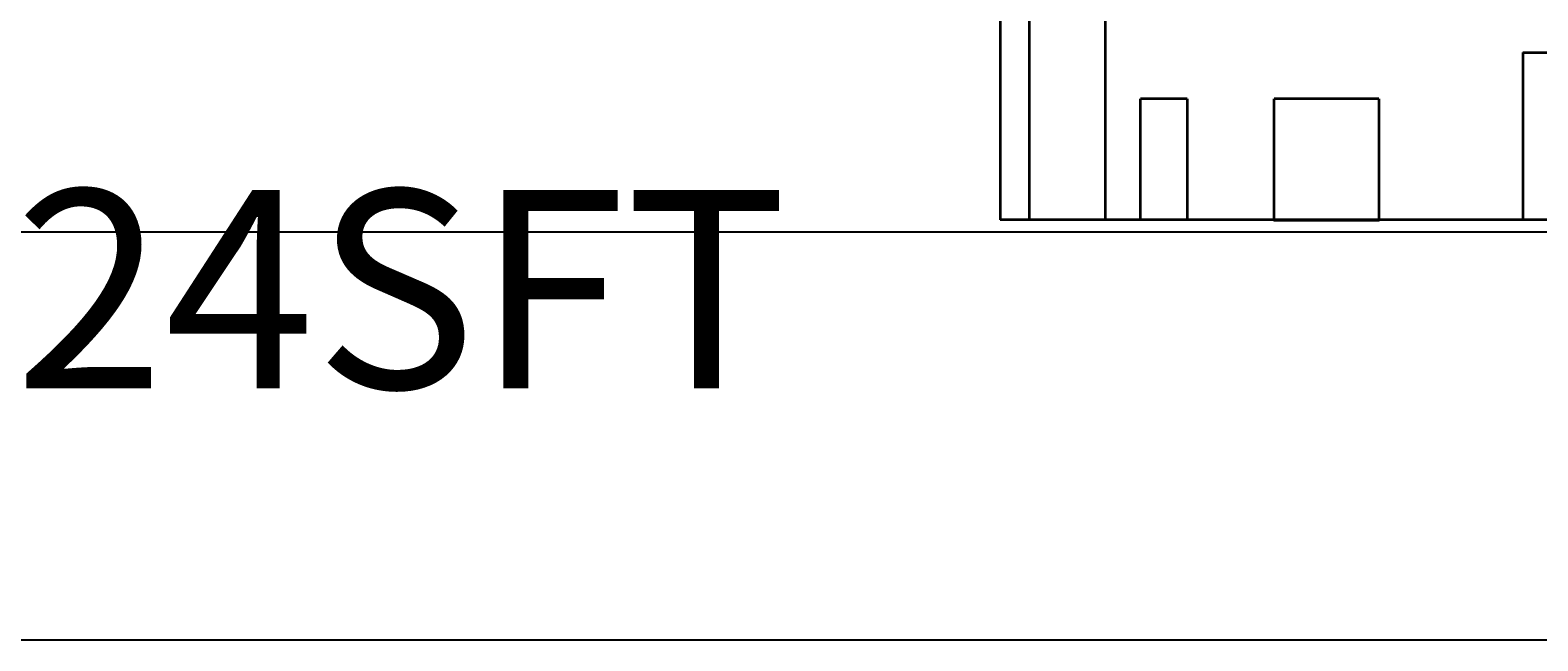
# Model space of a CAD drawing. Units: millimetres. Extents: x 27017497 to 27018854, y 7058029 to 7059154.
# Tile 18 of 91: x 27017651 to 27017886, y 7058029 to 7058124. Entities that reach past the tile are written whole.
import ezdxf

# ---------------------------------------------------------------- set-up
doc = ezdxf.new("R2010")
doc.units = ezdxf.units.MM
for name, color, linetype, lineweight in [('A-ANNO-DIMS', 2, 'Continuous', 18), ('A-AREA-IDEN', 7, 'Continuous', 18), ('A-WALL', 7, 'Continuous', 35)]:
    doc.layers.add(name, color=color, linetype=linetype, lineweight=lineweight)
doc.styles.get("Standard").update_dxf_attribs({"font": 'arial.ttf'})
doc.dimstyles.get("Standard").update_dxf_attribs({"dimtxt": 0.18, "dimasz": 0.18, "dimexe": 0.18, "dimexo": 0.0625, "dimgap": 0.09, "dimtad": 0, "dimtih": 1, "dimtoh": 1, "dimdec": 4, "dimzin": 0, "dimdsep": 46, "dimtxsty": 'Standard', "dimcen": 0.09, "dimadec": 0, "dimazin": 0, "dimtfac": 1, "dimtdec": 4, "dimtofl": 0, "dimtmove": 0, "dimatfit": 3, "dimfxl": 1, "dimtolj": 1, "dimtzin": 0, "dimarcsym": 0})

# ---------------------------------------------------------------- blocks, each defined once
blk = doc.blocks.new('*D47')
at = {"layer": 'A-ANNO-DIMS', "color": 0, "lineweight": -2, "transparency": 16777216}
for p, q in [((27017561.17, 7058294.35), (27017561.17, 7058028.6)), ((27018790.61, 7058294.35), (27018790.61, 7058028.6)), ((27017561.35, 7058028.78), (27018175.43, 7058028.78)), ((27018790.43, 7058028.78), (27018176.34, 7058028.78))]:
    blk.add_line(p, q, dxfattribs=at)
at = {"layer": 'A-ANNO-DIMS', "color": 0, "transparency": 16777216}
for points in [[(27017561.35, 7058028.81), (27017561.35, 7058028.75), (27017561.17, 7058028.78)], [(27018790.43, 7058028.81), (27018790.43, 7058028.75), (27018790.61, 7058028.78)]]:
    blk.add_solid(points, dxfattribs=at)
at = {"layer": 'Defpoints', "color": 0, "transparency": 16777216}
for p in [(27017561.17, 7058294.41), (27018790.61, 7058294.41), (27018790.61, 7058028.78)]:
    blk.add_point(p, dxfattribs=at)
at = {"layer": 'A-ANNO-DIMS', "color": 0, "transparency": 16777216, "insert": (27018175.89, 7058028.78), "char_height": 0.18, "attachment_point": 5}
blk.add_mtext('\\A1;1229.4', dxfattribs=at)
blk = doc.blocks.new('*D48')
at = {"layer": 'A-ANNO-DIMS', "color": 0, "lineweight": -2, "transparency": 16777216}
for p, q in [((27018463.5, 7058622.91), (27017497.54, 7058622.91)), ((27017497.72, 7058622.73), (27017497.72, 7058357.75)), ((27017497.72, 7058092.41), (27017497.72, 7058357.39)), ((27018555.13, 7058092.23), (27017497.54, 7058092.23))]:
    blk.add_line(p, q, dxfattribs=at)
at = {"layer": 'A-ANNO-DIMS', "color": 0, "transparency": 16777216}
for points in [[(27017497.69, 7058622.73), (27017497.75, 7058622.73), (27017497.72, 7058622.91)], [(27017497.69, 7058092.41), (27017497.75, 7058092.41), (27017497.72, 7058092.23)]]:
    blk.add_solid(points, dxfattribs=at)
at = {"layer": 'Defpoints', "color": 0, "transparency": 16777216}
for p in [(27018463.56, 7058622.91), (27017497.72, 7058092.23), (27018555.19, 7058092.23)]:
    blk.add_point(p, dxfattribs=at)
at = {"layer": 'A-ANNO-DIMS', "color": 0, "transparency": 16777216, "insert": (27017497.72, 7058357.57), "char_height": 0.18, "attachment_point": 5}
blk.add_mtext('\\A1;530.7', dxfattribs=at)

msp = doc.modelspace()

# ---------------------------------------------------------------- linework, layer by layer
at = {"layer": 'A-WALL'}
for p, q in [((27017802.166, 7058180.965), (27017802.166, 7058094.141)), ((27017806.666, 7058181.164), (27017806.666, 7058094.141)), ((27017818.555, 7058094.141), (27017818.555, 7058126.681)), ((27017883.582, 7058120.17), (27017883.582, 7058094.141)), ((27017883.582, 7058120.17), (27017901.33, 7058120.17)), ((27017831.311, 7058112.963), (27017824.003, 7058112.963)), ((27017861.131, 7058112.963), (27017844.853, 7058112.963)), ((27017892.582, 7058094.141), (27017802.166, 7058094.141))]:
    msp.add_line(p, q, dxfattribs=at)
for points in [[(27017831.311, 7058112.963), (27017831.311, 7058094.141), (27017824.003, 7058094.141), (27017824.003, 7058112.963)], [(27017861.131, 7058112.963), (27017861.131, 7058094.054), (27017844.853, 7058094.054), (27017844.853, 7058112.963)]]:
    msp.add_lwpolyline(points, dxfattribs=at)

# ---------------------------------------------------------------- texts
at = {"layer": 'A-AREA-IDEN'}
msp.add_text('1824SFT', height=30.9043, dxfattribs=at).set_placement((27017601.779, 7058067.907))

# ---------------------------------------------------------------- dimensions: what is measured, and where the dimension line sits
at = {"layer": 'A-ANNO-DIMS'}
dim = msp.add_linear_dim(base=(27017497.716, 7058092.23), p1=(27018463.561, 7058622.912), p2=(27018555.192, 7058092.23), angle=90, dimstyle='Standard', override={"dimdec": 1, "dimlfac": 1, "dimrnd": 0, "dimzin": 0, "dimdsep": 46, "dimlunit": 2}, dxfattribs=at)
dim.commit()
dim.dimension.update_dxf_attribs({"geometry": '*D48', "text_midpoint": (27017497.716, 7058357.571)})
dim = msp.add_linear_dim(base=(27018790.606, 7058028.78), p1=(27017561.166, 7058294.412), p2=(27018790.606, 7058294.412), dimstyle='Standard', override={"dimdec": 1, "dimlfac": 1, "dimrnd": 0, "dimzin": 0, "dimdsep": 46, "dimlunit": 2}, dxfattribs=at)
dim.commit()
dim.dimension.update_dxf_attribs({"geometry": '*D47', "text_midpoint": (27018175.886, 7058028.78)})

doc.saveas('drawing.dxf')
